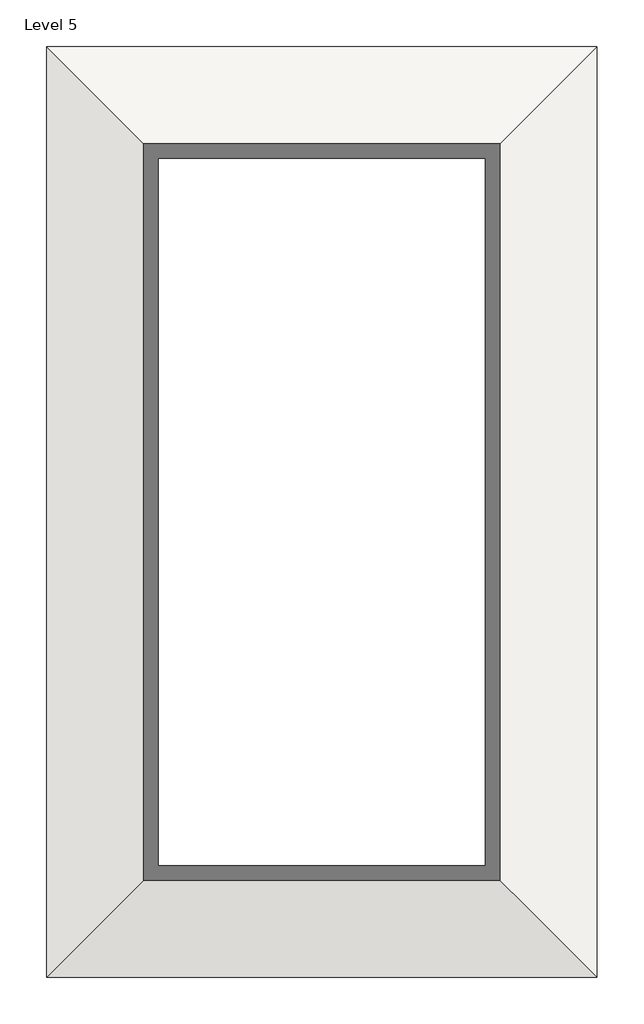
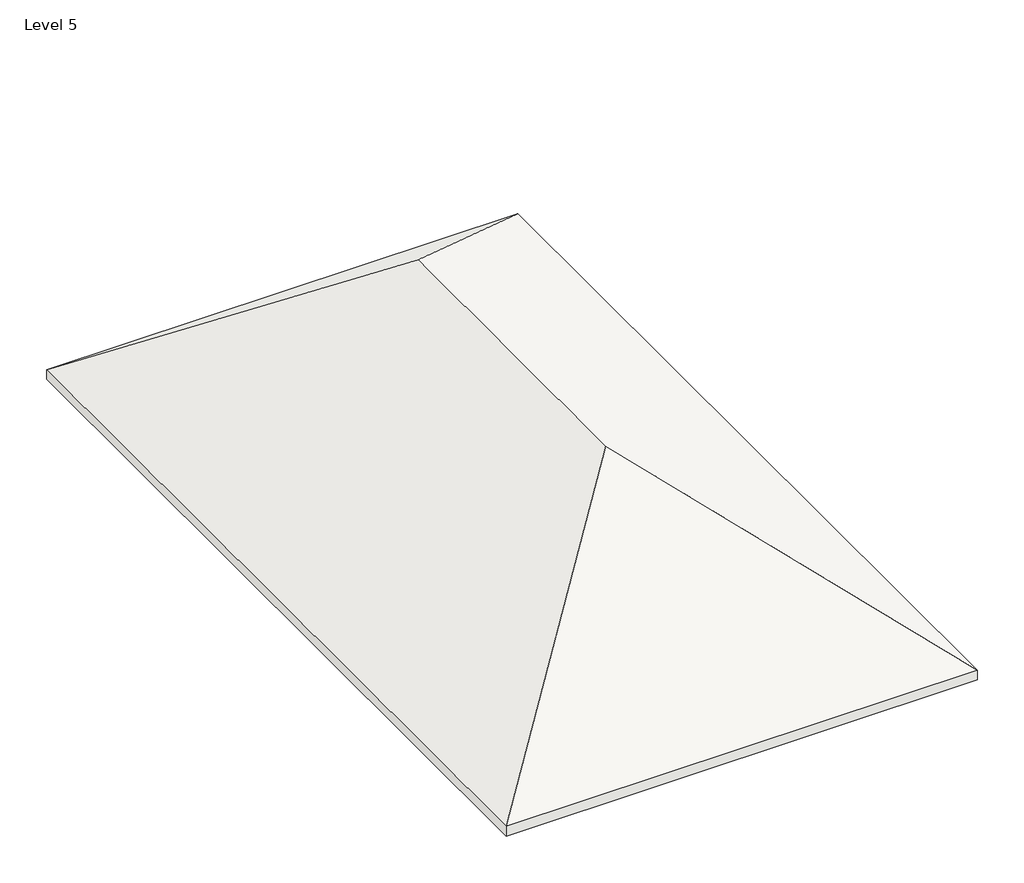
# One storey: 1 roof.
"""IFC4 building model written with IfcOpenShell, lengths in millimetres."""

from ifc_helpers import new_model, si_unit, origin, place, context, project, spatial, faceted_brep, element, save

model = new_model("IFC4")

# Units and contexts
model_context = context("Model", 3, world=origin())
ifc_project = project(units=[si_unit("LENGTHUNIT", "METRE", prefix="MILLI")], contexts=[model_context])

# Site, building, storey
site = spatial("IfcSite", under=ifc_project)
building = spatial("IfcBuilding", under=site)
storey = spatial("IfcBuildingStorey", under=building, Name="Level 5", Elevation=9601.2)

# Roof
placement = place(None, origin())
element("IfcRoof", 1, ObjectType="Generic - 12\"", at=placement, inside=storey, context=model_context, shape_type="Brep", body=[
    faceted_brep([(3164.3584916, 8005.7935985, 9448.8), (-1255.2415084, 3586.1935985, 12763.5), (-5674.8415084, 8005.7935985, 9448.8), (-1255.2415084, -2509.8064015, 12763.5), (-5674.8415084, -6929.4064015, 9448.8), (3164.3584916, -6929.4064015, 9448.8), (3164.3584916, 8005.7935985, 9639.3), (-5674.8415084, 8005.7935985, 9639.3), (-1255.2415084, 3586.1935985, 12954.0), (-5674.8415084, -6929.4064015, 9639.3), (-1255.2415084, -2509.8064015, 12954.0), (3164.3584916, -6929.4064015, 9639.3)], [[[0, 1, 2]], [[2, 1, 3, 4]], [[4, 3, 5]], [[1, 0, 5, 3]], [[6, 7, 8]], [[7, 9, 10, 8]], [[9, 11, 10]], [[6, 8, 10, 11]], [[2, 7, 6, 0]], [[4, 9, 7, 2]], [[5, 11, 9, 4]], [[0, 6, 11, 5]]]),
])

save(model, "model.ifc")

# Revit data of these elements
# Type "Generic - 12\""
#   Assembly Code = "B1020"
#   Layers, outside or top first: 0' - 6" no material (function 1)
# Element 1 (IfcRoof, "Generic - 12\"")
#   built-in parameter 1001705 = 42.5 (stored number, unit not read)
#   built-in parameter 1001701 = -0.5 (stored number, unit not read)
#   built-in parameter 1001710 = 33615
#   Phase Created = New Construction
#   Materials on its faces: "Cherry", "sheets", "Default Roof", "Brick, Common"
# Materials
#   "Cherry": class "Wood", colour RGB 226 177 128, transparency 0, Description = "Prunus Serotina", Cost = 0
#   "sheets": colour RGB 200 195 176, transparency 0, Cost = 0
#   "Default Roof": colour RGB 88 101 114, transparency 0, Cost = 0
#   "Brick, Common": class "Masonry", colour RGB 170 98 104, transparency 0, Description = "Common brick", Cost = 0
